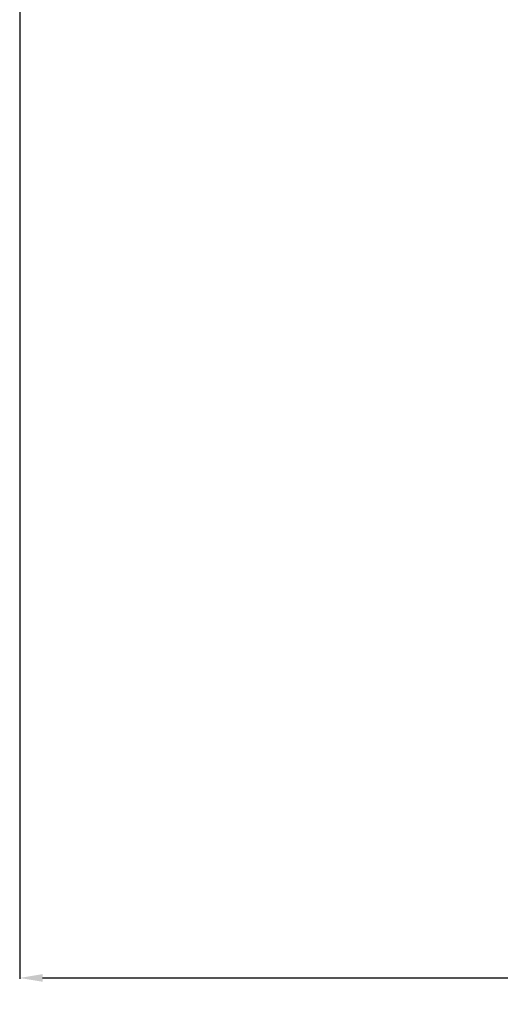
# Model space of a CAD drawing. Units: millimetres. Extents: x 0 to 2267, y 0 to 1823.
# Tile 1 of 256: x 1506 to 1590, y 902 to 1074. Entities that reach past the tile are written whole.
import ezdxf

# ---------------------------------------------------------------- set-up
doc = ezdxf.new("R2010")
doc.units = ezdxf.units.MM
doc.header["$MEASUREMENT"] = 0
doc.layers.add('M-DIMS', color=2, linetype='Continuous', lineweight=25)
doc.styles.get("Standard").update_dxf_attribs({"font": 'arial.ttf'})
doc.dimstyles.get("Standard").update_dxf_attribs({"dimtxt": 7, "dimasz": 4, "dimexe": 0.18, "dimexo": 0.0625, "dimgap": 0.09, "dimtad": 0, "dimdec": 0, "dimzin": 0, "dimdsep": 46, "dimtxsty": 'Standard', "dimcen": 0.09, "dimadec": 0, "dimazin": 0, "dimtfac": 1, "dimtdec": 0, "dimtofl": 0, "dimtmove": 0, "dimatfit": 3, "dimfxl": 1, "dimtolj": 1, "dimtzin": 0, "dimarcsym": 0})

# ---------------------------------------------------------------- blocks, each defined once
blk = doc.blocks.new('*D2')
at = {"layer": 'Defpoints', "color": 0, "transparency": 16777216}
for p in [(1505.93, 1077.42), (1930.93, 1077.42), (1930.93, 906.79)]:
    blk.add_point(p, dxfattribs=at)
at = {"layer": 'M-DIMS', "color": 0, "lineweight": -2, "transparency": 16777216}
for p, q in [((1505.93, 1077.35), (1505.93, 906.61)), ((1930.93, 1077.35), (1930.93, 906.61)), ((1509.93, 906.79), (1710.44, 906.79)), ((1926.93, 906.79), (1726.42, 906.79))]:
    blk.add_line(p, q, dxfattribs=at)
at = {"layer": 'M-DIMS', "color": 0, "transparency": 16777216}
for points in [[(1509.93, 907.45), (1509.93, 906.12), (1505.93, 906.79)], [(1926.93, 907.45), (1926.93, 906.12), (1930.93, 906.79)]]:
    blk.add_solid(points, dxfattribs=at)
at = {"layer": 'M-DIMS', "color": 0, "transparency": 16777216, "insert": (1718.43, 906.79), "char_height": 7, "attachment_point": 5}
blk.add_mtext('\\A1;425', dxfattribs=at)

msp = doc.modelspace()

# ---------------------------------------------------------------- dimensions: what is measured, and where the dimension line sits
at = {"layer": 'M-DIMS'}
dim = msp.add_linear_dim(base=(1930.929, 906.787), p1=(1505.929, 1077.417), p2=(1930.929, 1077.417), dimstyle='Standard', override={"dimclrd": 0, "dimclre": 0, "dimclrt": 0}, dxfattribs=at)
dim.commit()
dim.dimension.update_dxf_attribs({"geometry": '*D2', "text_midpoint": (1718.429, 906.787)})

doc.saveas('drawing.dxf')
